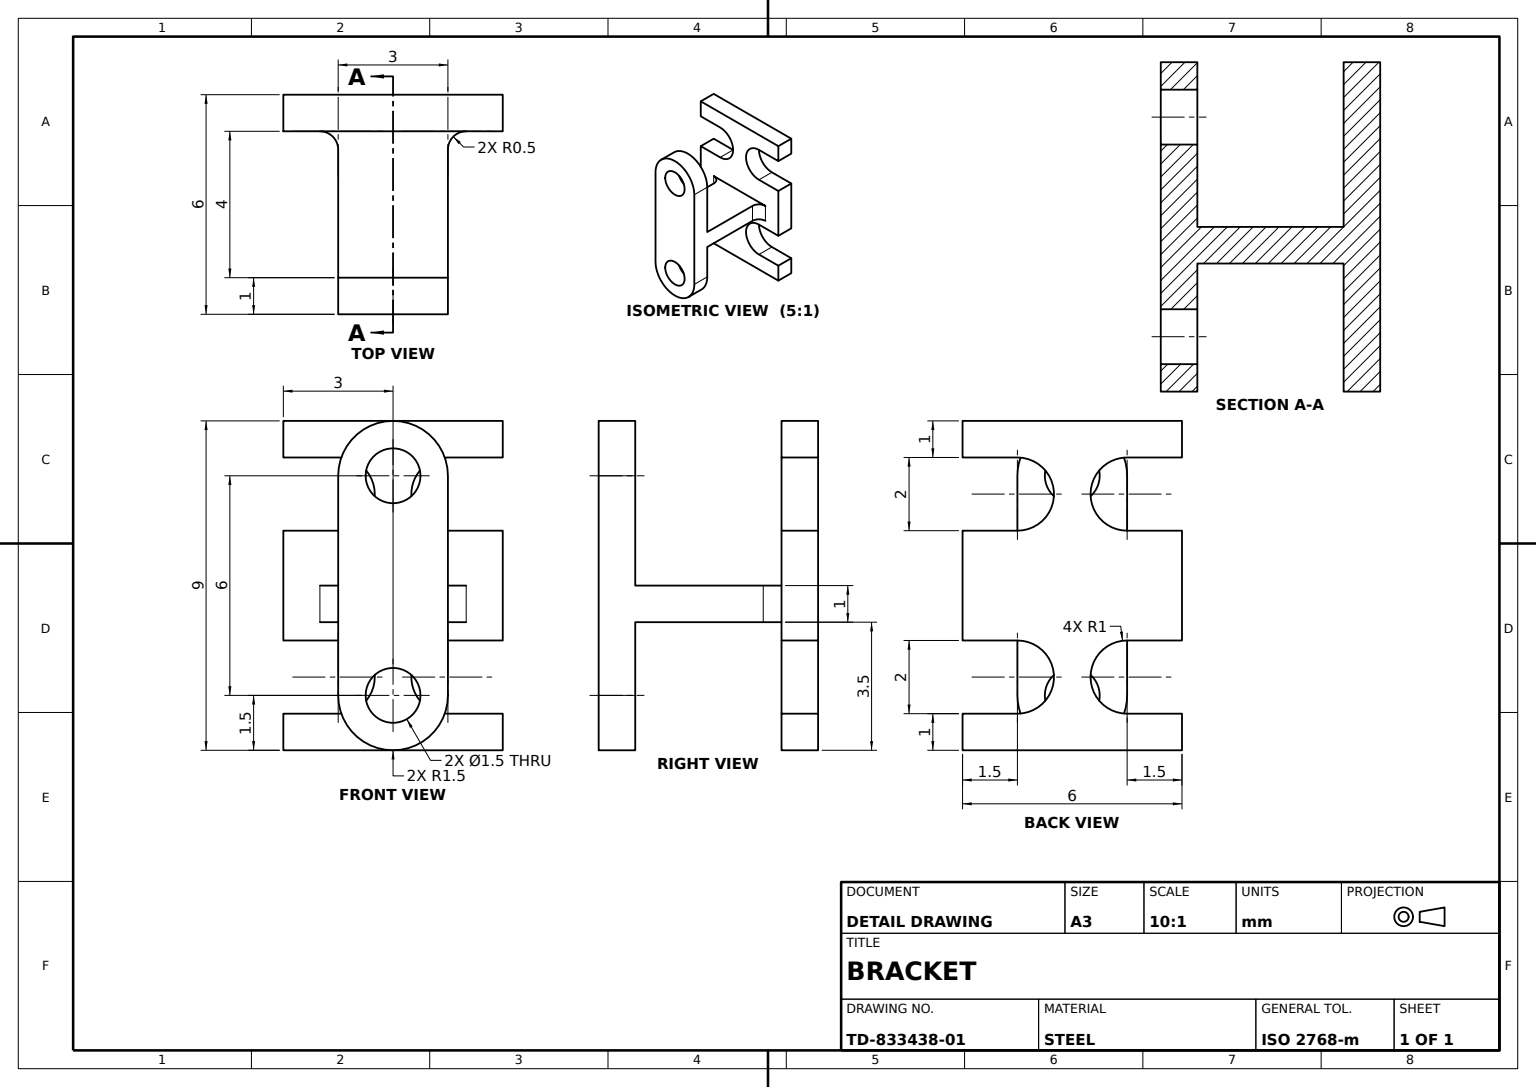
from build123d import *

# Parameters (mm, degrees)
BASE_PLATE_SKETCH_W  = 6
BASE_PLATE_SKETCH_H  = 6
BASE_PLATE_DEPTH     = 1
UPPER_PAD_SKETCH_W   = 6
UPPER_PAD_SKETCH_H   = 1
UPPER_PAD_DEPTH      = 1.5
LOWER_PAD_SKETCH_W   = 6
LOWER_PAD_SKETCH_H   = 1
LOWER_PAD_DEPTH      = 1.5
NOTCH_CUTS_DEPTH     = 1.5
STEM_SKETCH_W        = 3
STEM_SKETCH_H        = 1
STEM_1X3_DEPTH       = 4
STEM_FILLET_R0_5_A_R = 0.5
STEM_FILLET_R0_5_B_R = 0.5
LUG_PLATE_SKETCH_R   = 0.75
LUG_PLATE_DEPTH      = 1


with BuildPart() as part:
    # Base Plate Sketch → Base Plate (new body)
    with BuildSketch(Plane.XY):
        Rectangle(BASE_PLATE_SKETCH_W, BASE_PLATE_SKETCH_H)
    extrude(amount=-BASE_PLATE_DEPTH)

    # Upper Pad Sketch → Upper Pad (add)
    with BuildSketch(Plane(origin=(0, 3, 0), x_dir=(1, 0, 0), z_dir=(0, 1, 0))):
        with Locations((0, 0.5)):
            Rectangle(UPPER_PAD_SKETCH_W, UPPER_PAD_SKETCH_H)
    extrude(amount=UPPER_PAD_DEPTH)

    # Lower Pad Sketch → Lower Pad (add)
    with BuildSketch(Plane.XZ.offset(3)):
        with Locations((0, -0.5)):
            Rectangle(LOWER_PAD_SKETCH_W, LOWER_PAD_SKETCH_H)
    extrude(amount=LOWER_PAD_DEPTH)

    # Notch Cut Sketch → Notch Cuts (cut)
    with BuildSketch(Plane.XY):
        with BuildLine():
            Line((-1.5, 3.5), (-3, 3.5))
            Line((-3, 3.5), (-3, 1.5))
            Line((-3, 1.5), (-1.5, 1.5))
            ThreePointArc((-1.5, 1.5), (-0.5, 2.5), (-1.5, 3.5))
        make_face()
        with BuildLine():
            Line((1.5, 3.5), (3, 3.5))
            Line((3, 3.5), (3, 1.5))
            Line((3, 1.5), (1.5, 1.5))
            ThreePointArc((1.5, 1.5), (0.5, 2.5), (1.5, 3.5))
        make_face()
        with BuildLine():
            Line((3, -1.5), (3, -3.5))
            Line((3, -3.5), (1.5, -3.5))
            ThreePointArc((1.5, -3.5), (0.5, -2.5), (1.5, -1.5))
            Line((1.5, -1.5), (3, -1.5))
        make_face()
        with BuildLine():
            Line((-1.5, -1.5), (-3, -1.5))
            Line((-3, -1.5), (-3, -3.5))
            Line((-3, -3.5), (-1.5, -3.5))
            ThreePointArc((-1.5, -3.5), (-0.5, -2.5), (-1.5, -1.5))
        make_face()
    extrude(amount=-NOTCH_CUTS_DEPTH, mode=Mode.SUBTRACT)

    # Stem Sketch → Stem 1x3 (add)
    with BuildSketch(Plane.XY):
        with Locations((0, -0.5)):
            Rectangle(STEM_SKETCH_W, STEM_SKETCH_H)
    extrude(amount=STEM_1X3_DEPTH)

    # Stem Fillet R0.5 A
    stem_fillet_r0_5_a_edges = [part.edges().sort_by_distance(p)[0] for p in [
        (1.5, -0.5, 0),
    ]]
    fillet(stem_fillet_r0_5_a_edges, radius=STEM_FILLET_R0_5_A_R)

    # Stem Fillet R0.5 B
    stem_fillet_r0_5_b_edges = [part.edges().sort_by_distance(p)[0] for p in [
        (-1.5, -0.5, 0),
    ]]
    fillet(stem_fillet_r0_5_b_edges, radius=STEM_FILLET_R0_5_B_R)

    # Lug Plate Sketch → Lug Plate (add)
    with BuildSketch(Plane.XY.offset(4)):
        with BuildLine():
            Line((1.5, 3), (1.5, -3))
            ThreePointArc((1.5, -3), (0, -4.5), (-1.5, -3))
            Line((-1.5, -3), (-1.5, 3))
            ThreePointArc((-1.5, 3), (0, 4.5), (1.5, 3))
        make_face()
        with Locations((0, 3)):
            Circle(LUG_PLATE_SKETCH_R, mode=Mode.SUBTRACT)
        with Locations((0, -3)):
            Circle(LUG_PLATE_SKETCH_R, mode=Mode.SUBTRACT)
    extrude(amount=LUG_PLATE_DEPTH)


solid = part.part
